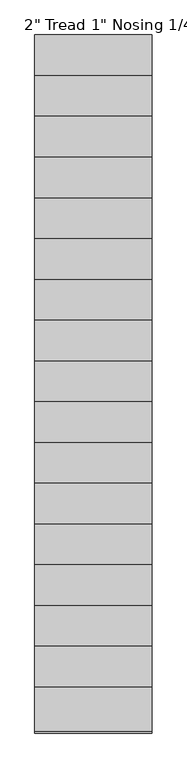
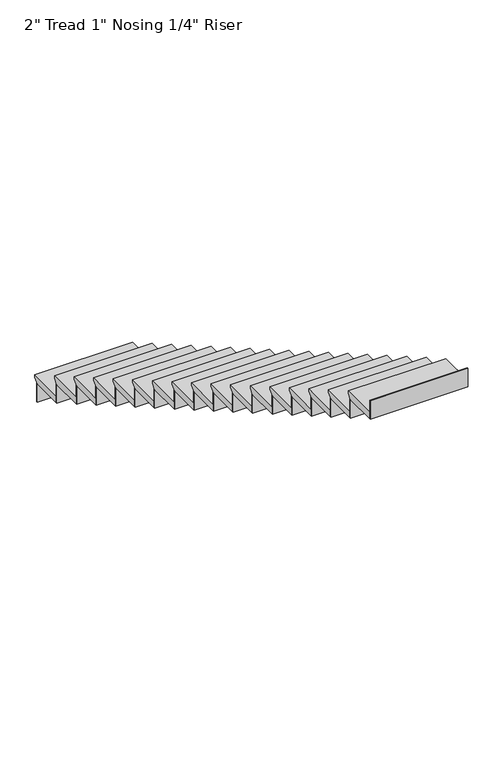
"""IFC4 building model written with IfcOpenShell, lengths in millimetres: stair flight geometry."""

from ifc_helpers import new_model, si_unit, frame, origin, place, context, project, spatial, polyline, outline, extrude, source, transform, mapped, element, save


def stair_flight_246ebb71(model_context):
    return source(origin(), model_context, "Body", "SweptSolid", [
        extrude(outline(polyline([(5740.7076853, 8032.75), (6020.1076853, 8032.75), (6020.1076853, 8013.7), (5994.7076853, 7988.3), (5994.7076853, 7981.95), (5740.7076853, 7981.95), (5740.7076853, 8032.75)])), frame((-6854.5155596, 0.0, 0.0), z_axis=(1.0, 0.0, 0.0), x_axis=(0.0, 1.0, 0.0)), (0.0, 0.0, 1.0), 731.52),
        extrude(outline(polyline([(-6854.5155596, 5988.3576853), (-6854.5155596, 5994.7076853), (-6122.9955596, 5994.7076853), (-6122.9955596, 5988.3576853), (-6854.5155596, 5988.3576853)])), frame((0.0, 0.0, 7835.9), z_axis=(0.0, 0.0, 1.0), x_axis=(1.0, 0.0, 0.0)), (0.0, 0.0, 1.0), 146.05),
        extrude(outline(polyline([(-6854.5155596, 5734.3576853), (-6854.5155596, 5740.7076853), (-6122.9955596, 5740.7076853), (-6122.9955596, 5734.3576853), (-6854.5155596, 5734.3576853)])), frame((0.0, 0.0, 7981.95), z_axis=(0.0, 0.0, 1.0), x_axis=(1.0, 0.0, 0.0)), (0.0, 0.0, 1.0), 146.05),
        extrude(outline(polyline([(5486.7076853, 8178.8), (5766.1076853, 8178.8), (5766.1076853, 8159.75), (5740.7076853, 8134.35), (5740.7076853, 8128.0), (5486.7076853, 8128.0), (5486.7076853, 8178.8)])), frame((-6854.5155596, 0.0, 0.0), z_axis=(1.0, 0.0, 0.0), x_axis=(0.0, 1.0, 0.0)), (0.0, 0.0, 1.0), 731.52),
        extrude(outline(polyline([(-6854.5155596, 5480.3576853), (-6854.5155596, 5486.7076853), (-6122.9955596, 5486.7076853), (-6122.9955596, 5480.3576853), (-6854.5155596, 5480.3576853)])), frame((0.0, 0.0, 8128.0), z_axis=(0.0, 0.0, 1.0), x_axis=(1.0, 0.0, 0.0)), (0.0, 0.0, 1.0), 146.05),
        extrude(outline(polyline([(5232.7076853, 8324.85), (5512.1076853, 8324.85), (5512.1076853, 8305.8), (5486.7076853, 8280.4), (5486.7076853, 8274.05), (5232.7076853, 8274.05), (5232.7076853, 8324.85)])), frame((-6854.5155596, 0.0, 0.0), z_axis=(1.0, 0.0, 0.0), x_axis=(0.0, 1.0, 0.0)), (0.0, 0.0, 1.0), 731.52),
        extrude(outline(polyline([(-6854.5155596, 5226.3576853), (-6854.5155596, 5232.7076853), (-6122.9955596, 5232.7076853), (-6122.9955596, 5226.3576853), (-6854.5155596, 5226.3576853)])), frame((0.0, 0.0, 8274.05), z_axis=(0.0, 0.0, 1.0), x_axis=(1.0, 0.0, 0.0)), (0.0, 0.0, 1.0), 146.05),
        extrude(outline(polyline([(4978.7076853, 8470.9), (5258.1076853, 8470.9), (5258.1076853, 8451.85), (5232.7076853, 8426.45), (5232.7076853, 8420.1), (4978.7076853, 8420.1), (4978.7076853, 8470.9)])), frame((-6854.5155596, 0.0, 0.0), z_axis=(1.0, 0.0, 0.0), x_axis=(0.0, 1.0, 0.0)), (0.0, 0.0, 1.0), 731.52),
        extrude(outline(polyline([(-6854.5155596, 4972.3576853), (-6854.5155596, 4978.7076853), (-6122.9955596, 4978.7076853), (-6122.9955596, 4972.3576853), (-6854.5155596, 4972.3576853)])), frame((0.0, 0.0, 8420.1), z_axis=(0.0, 0.0, 1.0), x_axis=(1.0, 0.0, 0.0)), (0.0, 0.0, 1.0), 146.05),
        extrude(outline(polyline([(4724.7076853, 8616.95), (5004.1076853, 8616.95), (5004.1076853, 8597.9), (4978.7076853, 8572.5), (4978.7076853, 8566.15), (4724.7076853, 8566.15), (4724.7076853, 8616.95)])), frame((-6854.5155596, 0.0, 0.0), z_axis=(1.0, 0.0, 0.0), x_axis=(0.0, 1.0, 0.0)), (0.0, 0.0, 1.0), 731.52),
        extrude(outline(polyline([(-6854.5155596, 4718.3576853), (-6854.5155596, 4724.7076853), (-6122.9955596, 4724.7076853), (-6122.9955596, 4718.3576853), (-6854.5155596, 4718.3576853)])), frame((0.0, 0.0, 8566.15), z_axis=(0.0, 0.0, 1.0), x_axis=(1.0, 0.0, 0.0)), (0.0, 0.0, 1.0), 146.05),
        extrude(outline(polyline([(4470.7076853, 8763.0), (4750.1076853, 8763.0), (4750.1076853, 8743.95), (4724.7076853, 8718.55), (4724.7076853, 8712.2), (4470.7076853, 8712.2), (4470.7076853, 8763.0)])), frame((-6854.5155596, 0.0, 0.0), z_axis=(1.0, 0.0, 0.0), x_axis=(0.0, 1.0, 0.0)), (0.0, 0.0, 1.0), 731.52),
        extrude(outline(polyline([(-6854.5155596, 4464.3576853), (-6854.5155596, 4470.7076853), (-6122.9955596, 4470.7076853), (-6122.9955596, 4464.3576853), (-6854.5155596, 4464.3576853)])), frame((0.0, 0.0, 8712.2), z_axis=(0.0, 0.0, 1.0), x_axis=(1.0, 0.0, 0.0)), (0.0, 0.0, 1.0), 146.05),
        extrude(outline(polyline([(4216.7076853, 8909.05), (4496.1076853, 8909.05), (4496.1076853, 8890.0), (4470.7076853, 8864.6), (4470.7076853, 8858.25), (4216.7076853, 8858.25), (4216.7076853, 8909.05)])), frame((-6854.5155596, 0.0, 0.0), z_axis=(1.0, 0.0, 0.0), x_axis=(0.0, 1.0, 0.0)), (0.0, 0.0, 1.0), 731.52),
        extrude(outline(polyline([(-6854.5155596, 4210.3576853), (-6854.5155596, 4216.7076853), (-6122.9955596, 4216.7076853), (-6122.9955596, 4210.3576853), (-6854.5155596, 4210.3576853)])), frame((0.0, 0.0, 8858.25), z_axis=(0.0, 0.0, 1.0), x_axis=(1.0, 0.0, 0.0)), (0.0, 0.0, 1.0), 146.05),
        extrude(outline(polyline([(3962.7076853, 9055.1), (4242.1076853, 9055.1), (4242.1076853, 9036.05), (4216.7076853, 9010.65), (4216.7076853, 9004.3), (3962.7076853, 9004.3), (3962.7076853, 9055.1)])), frame((-6854.5155596, 0.0, 0.0), z_axis=(1.0, 0.0, 0.0), x_axis=(0.0, 1.0, 0.0)), (0.0, 0.0, 1.0), 731.52),
        extrude(outline(polyline([(-6854.5155596, 3956.3576853), (-6854.5155596, 3962.7076853), (-6122.9955596, 3962.7076853), (-6122.9955596, 3956.3576853), (-6854.5155596, 3956.3576853)])), frame((0.0, 0.0, 9004.3), z_axis=(0.0, 0.0, 1.0), x_axis=(1.0, 0.0, 0.0)), (0.0, 0.0, 1.0), 146.05),
        extrude(outline(polyline([(3708.7076853, 9201.15), (3988.1076853, 9201.15), (3988.1076853, 9182.1), (3962.7076853, 9156.7), (3962.7076853, 9150.35), (3708.7076853, 9150.35), (3708.7076853, 9201.15)])), frame((-6854.5155596, 0.0, 0.0), z_axis=(1.0, 0.0, 0.0), x_axis=(0.0, 1.0, 0.0)), (0.0, 0.0, 1.0), 731.52),
        extrude(outline(polyline([(-6854.5155596, 3702.3576853), (-6854.5155596, 3708.7076853), (-6122.9955596, 3708.7076853), (-6122.9955596, 3702.3576853), (-6854.5155596, 3702.3576853)])), frame((0.0, 0.0, 9150.35), z_axis=(0.0, 0.0, 1.0), x_axis=(1.0, 0.0, 0.0)), (0.0, 0.0, 1.0), 146.05),
        extrude(outline(polyline([(3454.7076853, 9347.2), (3734.1076853, 9347.2), (3734.1076853, 9328.15), (3708.7076853, 9302.75), (3708.7076853, 9296.4), (3454.7076853, 9296.4), (3454.7076853, 9347.2)])), frame((-6854.5155596, 0.0, 0.0), z_axis=(1.0, 0.0, 0.0), x_axis=(0.0, 1.0, 0.0)), (0.0, 0.0, 1.0), 731.52),
        extrude(outline(polyline([(-6854.5155596, 3448.3576853), (-6854.5155596, 3454.7076853), (-6122.9955596, 3454.7076853), (-6122.9955596, 3448.3576853), (-6854.5155596, 3448.3576853)])), frame((0.0, 0.0, 9296.4), z_axis=(0.0, 0.0, 1.0), x_axis=(1.0, 0.0, 0.0)), (0.0, 0.0, 1.0), 146.05),
        extrude(outline(polyline([(3200.7076853, 9493.25), (3480.1076853, 9493.25), (3480.1076853, 9474.2), (3454.7076853, 9448.8), (3454.7076853, 9442.45), (3200.7076853, 9442.45), (3200.7076853, 9493.25)])), frame((-6854.5155596, 0.0, 0.0), z_axis=(1.0, 0.0, 0.0), x_axis=(0.0, 1.0, 0.0)), (0.0, 0.0, 1.0), 731.52),
        extrude(outline(polyline([(-6854.5155596, 3194.3576853), (-6854.5155596, 3200.7076853), (-6122.9955596, 3200.7076853), (-6122.9955596, 3194.3576853), (-6854.5155596, 3194.3576853)])), frame((0.0, 0.0, 9442.45), z_axis=(0.0, 0.0, 1.0), x_axis=(1.0, 0.0, 0.0)), (0.0, 0.0, 1.0), 146.05),
        extrude(outline(polyline([(2946.7076853, 9639.3), (3226.1076853, 9639.3), (3226.1076853, 9620.25), (3200.7076853, 9594.85), (3200.7076853, 9588.5), (2946.7076853, 9588.5), (2946.7076853, 9639.3)])), frame((-6854.5155596, 0.0, 0.0), z_axis=(1.0, 0.0, 0.0), x_axis=(0.0, 1.0, 0.0)), (0.0, 0.0, 1.0), 731.52),
        extrude(outline(polyline([(-6854.5155596, 2940.3576853), (-6854.5155596, 2946.7076853), (-6122.9955596, 2946.7076853), (-6122.9955596, 2940.3576853), (-6854.5155596, 2940.3576853)])), frame((0.0, 0.0, 9588.5), z_axis=(0.0, 0.0, 1.0), x_axis=(1.0, 0.0, 0.0)), (0.0, 0.0, 1.0), 146.05),
        extrude(outline(polyline([(2692.7076853, 9785.35), (2972.1076853, 9785.35), (2972.1076853, 9766.3), (2946.7076853, 9740.9), (2946.7076853, 9734.55), (2692.7076853, 9734.55), (2692.7076853, 9785.35)])), frame((-6854.5155596, 0.0, 0.0), z_axis=(1.0, 0.0, 0.0), x_axis=(0.0, 1.0, 0.0)), (0.0, 0.0, 1.0), 731.52),
        extrude(outline(polyline([(-6854.5155596, 2686.3576853), (-6854.5155596, 2692.7076853), (-6122.9955596, 2692.7076853), (-6122.9955596, 2686.3576853), (-6854.5155596, 2686.3576853)])), frame((0.0, 0.0, 9734.55), z_axis=(0.0, 0.0, 1.0), x_axis=(1.0, 0.0, 0.0)), (0.0, 0.0, 1.0), 146.05),
        extrude(outline(polyline([(2438.7076853, 9931.4), (2718.1076853, 9931.4), (2718.1076853, 9912.35), (2692.7076853, 9886.95), (2692.7076853, 9880.6), (2438.7076853, 9880.6), (2438.7076853, 9931.4)])), frame((-6854.5155596, 0.0, 0.0), z_axis=(1.0, 0.0, 0.0), x_axis=(0.0, 1.0, 0.0)), (0.0, 0.0, 1.0), 731.52),
        extrude(outline(polyline([(-6854.5155596, 2432.3576853), (-6854.5155596, 2438.7076853), (-6122.9955596, 2438.7076853), (-6122.9955596, 2432.3576853), (-6854.5155596, 2432.3576853)])), frame((0.0, 0.0, 9880.6), z_axis=(0.0, 0.0, 1.0), x_axis=(1.0, 0.0, 0.0)), (0.0, 0.0, 1.0), 146.05),
        extrude(outline(polyline([(2184.7076853, 10077.45), (2464.1076853, 10077.45), (2464.1076853, 10058.4), (2438.7076853, 10033.0), (2438.7076853, 10026.65), (2184.7076853, 10026.65), (2184.7076853, 10077.45)])), frame((-6854.5155596, 0.0, 0.0), z_axis=(1.0, 0.0, 0.0), x_axis=(0.0, 1.0, 0.0)), (0.0, 0.0, 1.0), 731.52),
        extrude(outline(polyline([(-6854.5155596, 2178.3576853), (-6854.5155596, 2184.7076853), (-6122.9955596, 2184.7076853), (-6122.9955596, 2178.3576853), (-6854.5155596, 2178.3576853)])), frame((0.0, 0.0, 10026.65), z_axis=(0.0, 0.0, 1.0), x_axis=(1.0, 0.0, 0.0)), (0.0, 0.0, 1.0), 146.05),
        extrude(outline(polyline([(1930.7076853, 10223.5), (2210.1076853, 10223.5), (2210.1076853, 10204.45), (2184.7076853, 10179.05), (2184.7076853, 10172.7), (1930.7076853, 10172.7), (1930.7076853, 10223.5)])), frame((-6854.5155596, 0.0, 0.0), z_axis=(1.0, 0.0, 0.0), x_axis=(0.0, 1.0, 0.0)), (0.0, 0.0, 1.0), 731.52),
        extrude(outline(polyline([(-6854.5155596, 1924.3576853), (-6854.5155596, 1930.7076853), (-6122.9955596, 1930.7076853), (-6122.9955596, 1924.3576853), (-6854.5155596, 1924.3576853)])), frame((0.0, 0.0, 10172.7), z_axis=(0.0, 0.0, 1.0), x_axis=(1.0, 0.0, 0.0)), (0.0, 0.0, 1.0), 146.05),
        extrude(outline(polyline([(-6854.5155596, 1670.3576853), (-6854.5155596, 1676.7076853), (-6122.9955596, 1676.7076853), (-6122.9955596, 1670.3576853), (-6854.5155596, 1670.3576853)])), frame((0.0, 0.0, 10318.75), z_axis=(0.0, 0.0, 1.0), x_axis=(1.0, 0.0, 0.0)), (0.0, 0.0, 1.0), 146.05),
        extrude(outline(polyline([(1676.7076853, 10369.55), (1956.1076853, 10369.55), (1956.1076853, 10350.5), (1930.7076853, 10325.1), (1930.7076853, 10318.75), (1676.7076853, 10318.75), (1676.7076853, 10369.55)])), frame((-6854.5155596, 0.0, 0.0), z_axis=(1.0, 0.0, 0.0), x_axis=(0.0, 1.0, 0.0)), (0.0, 0.0, 1.0), 731.52),
    ])


if __name__ == "__main__":
    model = new_model("IFC4")
    model_context = context("Model", 3, world=origin())
    ifc_project = project(units=[si_unit("LENGTHUNIT", "METRE", prefix="MILLI")], contexts=[model_context])
    site = spatial("IfcSite", under=ifc_project)
    building = spatial("IfcBuilding", under=site)
    placement = place(None, origin())
    stair_flight_shape = stair_flight_246ebb71(model_context)
    element("IfcStairFlight", 1, ObjectType="2\" Tread 1\" Nosing 1/4\" Riser", at=placement, inside=building, context=model_context, shape_type="MappedRepresentation", body=[
        mapped(stair_flight_shape, transform((0.0, 0.0, 0.0), x_axis=(1.0, 0.0, 0.0), y_axis=(0.0, 1.0, 0.0), z_axis=(0.0, 0.0, 1.0))),
    ])
    save(model, "model.ifc")
